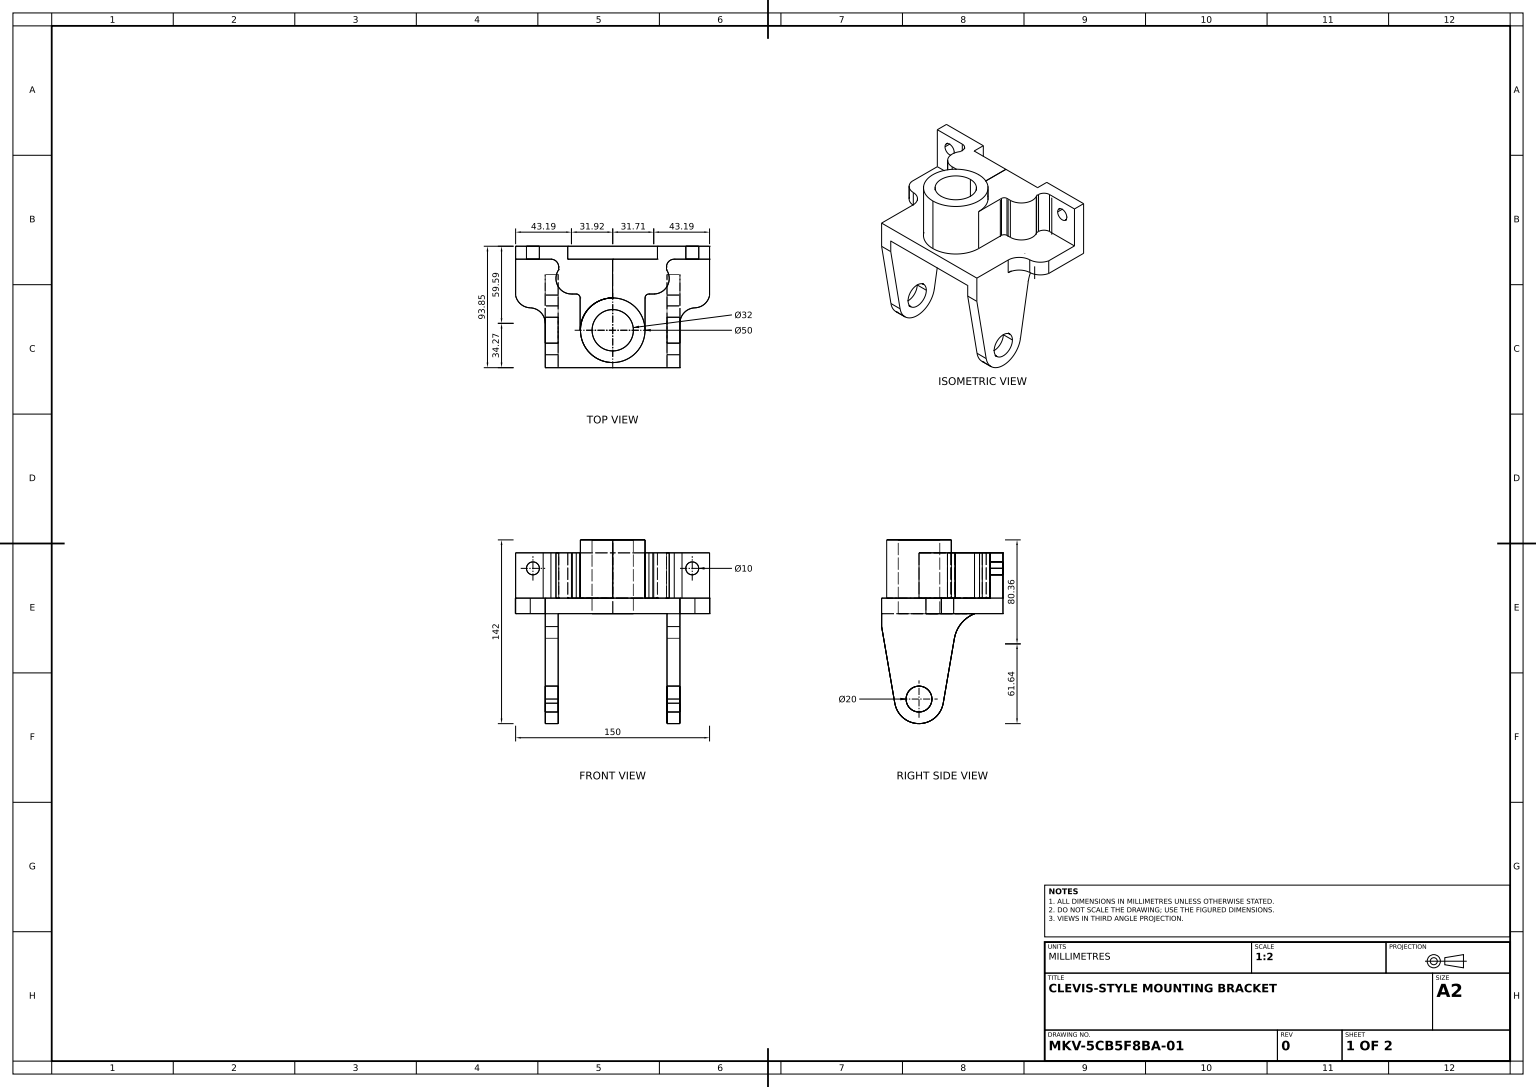
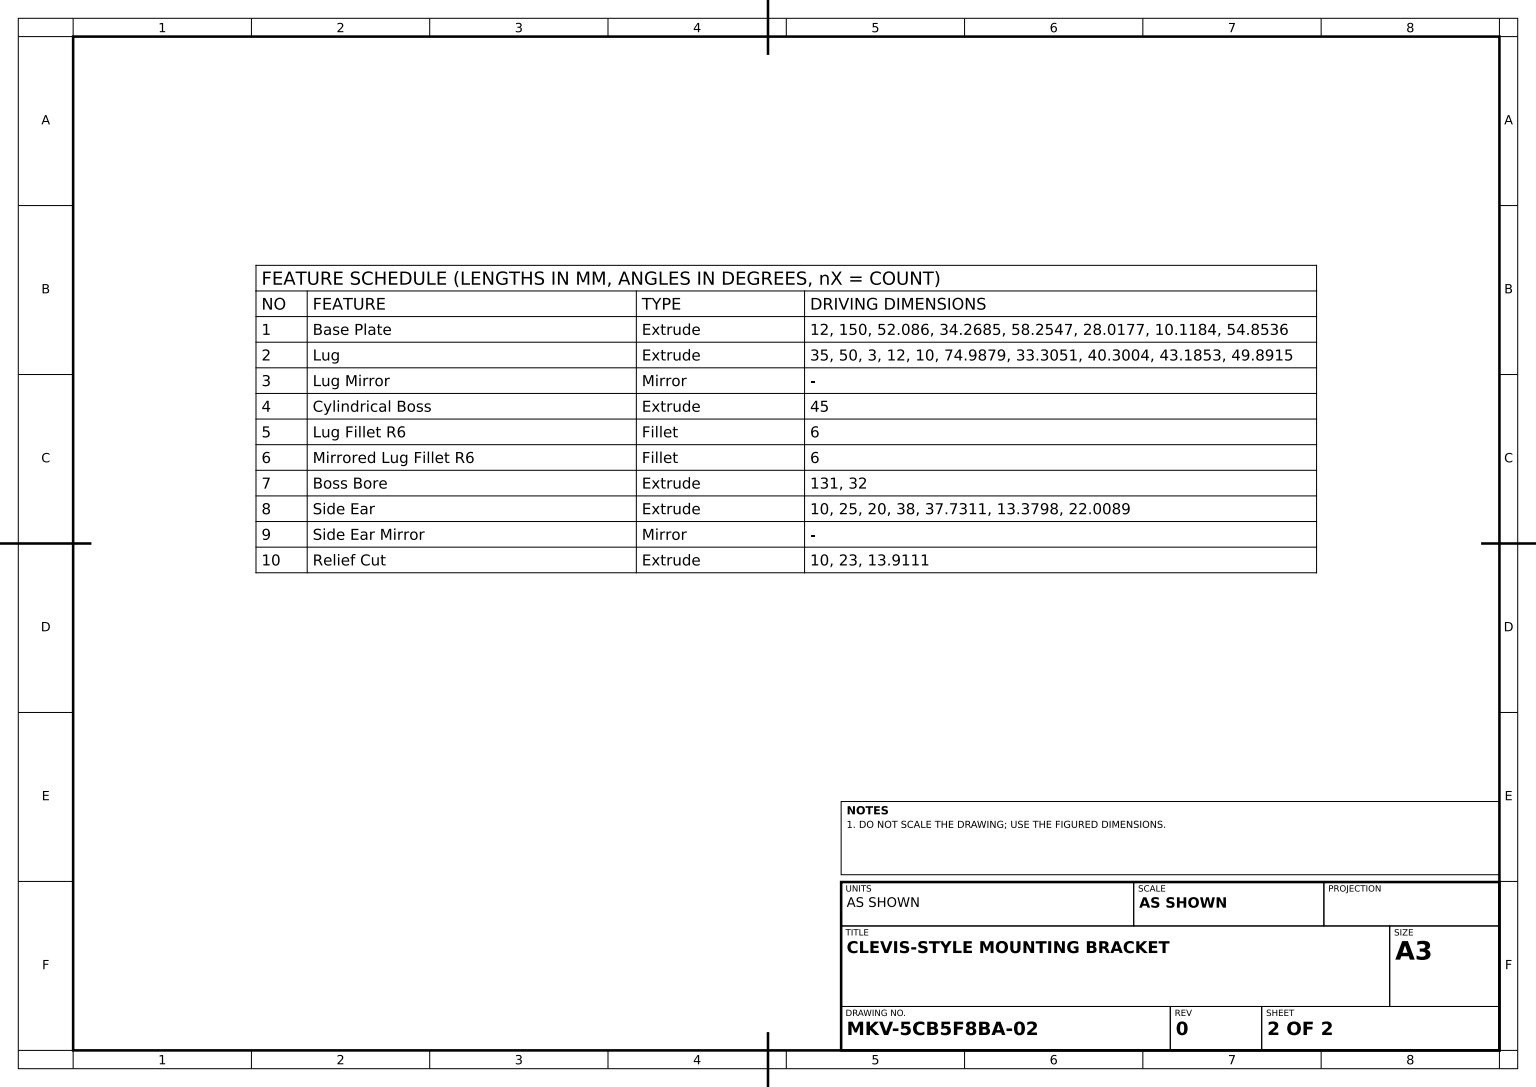
from build123d import *

# Parameters (mm, degrees)
BASE_PLATE_DEPTH         = 12
LUG_DEPTH                = 35
BOSS_SKETCH_R            = 25
CYLINDRICAL_BOSS_DEPTH   = 45
LUG_FILLET_R6_R          = 6
MIRRORED_LUG_FILLET_R6_R = 6
BOSS_BORE_SKETCH_R       = 16
BOSS_BORE_DEPTH          = 131
SIDE_EAR_SKETCH_R        = 10.000000003
SIDE_EAR_DEPTH           = 10
RELIEF_CUT_SKETCH_R      = 5
RELIEF_CUT_DEPTH         = 10


with BuildPart() as part:
    # Base Plate Sketch → Base Plate (new body)
    with BuildSketch(Plane(origin=(0, 0, 0), x_dir=(1, 0, 0), z_dir=(0, 1, 0))):
        with BuildLine():
            Line((0, 0), (52.086042587, 0))
            Line((52.086042587, 0), (52.086042587, 34.268491931))
            ThreePointArc((52.086042587, 34.268491931), (55.457925039, 42.608491187), (63.678640518, 46.261574252))
            ThreePointArc((63.678640518, 46.261574252), (70.963844757, 49.044672415), (75, 55.717699243))
            Line((75, 55.717699243), (75, 83.735383518))
            Line((75, 83.735383518), (75, 93.85377774))
            Line((75, 93.85377774), (20.146433568, 93.85377774))
            Line((20.146433568, 93.85377774), (-75, 93.85377774))
            Line((-75, 93.85377774), (-75, 83.735383518))
            Line((-75, 83.735383518), (-75, 55.717699243))
            ThreePointArc((-75, 55.717699243), (-70.963844757, 49.044672415), (-63.678640518, 46.261574252))
            ThreePointArc((-63.678640518, 46.261574252), (-55.457925039, 42.608491187), (-52.086042587, 34.268491931))
            Line((-52.086042587, 34.268491931), (-52.086042587, 0))
            Line((-52.086042587, 0), (0, 0))
        make_face()
    extrude(amount=BASE_PLATE_DEPTH)

    # Lug Sketch → Lug (add)
    with BuildSketch(Plane(origin=(0, 12, 0), x_dir=(1, 0, 0), z_dir=(0, 1, 0))):
        with BuildLine():
            ThreePointArc((0.048175719, 53.923822509), (17.764829386, 46.622880149), (25.108500916, 28.923895292))
            Line((25.108500916, 28.923895292), (25.108500916, 53.923895292))
            ThreePointArc((25.108500916, 53.923895292), (25.987180573, 56.045215635), (28.108500916, 56.923895292))
            Line((28.108500916, 56.923895292), (31.814716412, 56.923895292))
            ThreePointArc((31.814716412, 56.923895292), (42.43838692, 63.34378553), (41.694924329, 75.734291134))
            Line((41.694924329, 75.734291134), (41.694924329, 83.85377774))
            Line((41.694924329, 83.85377774), (75, 83.85377774))
            Line((75, 83.85377774), (75, 93.85377774))
            Line((75, 93.85377774), (41.694924329, 93.85377774))
            Line((41.694924329, 93.85377774), (34.699589824, 93.85377774))
            Line((34.699589824, 93.85377774), (34.699589824, 83.85377774))
            Line((34.699589824, 83.85377774), (0.012065057, 83.85377774))
            Line((0.012065057, 83.85377774), (0.048175719, 53.923822509))
        make_face()
    lug = extrude(amount=LUG_DEPTH)

    # Lug Mirror: Lug across plane
    add(lug.mirror(Plane(origin=(0, 0, 0), x_dir=(0, 0, 1), z_dir=(1, 0, 0))))

    # Boss Sketch → Cylindrical Boss (add)
    with BuildSketch(Plane(origin=(0, 12, 0), x_dir=(1, 0, 0), z_dir=(0, 1, 0))):
        with Locations(Location((0.108500916, 28.923895292, 0), (0, 0, 90.138255303))):
            Circle(BOSS_SKETCH_R)
    extrude(amount=CYLINDRICAL_BOSS_DEPTH)

    # Lug Fillet R6
    lug_fillet_r6_edges = [part.edges().sort_by_distance(p)[0] for p in [
        (41.694924329, 29.5, -83.85377774),
    ]]
    fillet(lug_fillet_r6_edges, radius=LUG_FILLET_R6_R)

    # Mirrored Lug Fillet R6
    mirrored_lug_fillet_r6_edges = [part.edges().sort_by_distance(p)[0] for p in [
        (-41.694924329, 29.5, -83.85377774),
    ]]
    fillet(mirrored_lug_fillet_r6_edges, radius=MIRRORED_LUG_FILLET_R6_R)

    # Boss Bore Sketch → Boss Bore (cut)
    with BuildSketch(Plane(origin=(0, 57, 0), x_dir=(1, 0, 0), z_dir=(0, 1, 0))):
        with Locations(Location((0.108500916, 28.923895292, 0), (0, 0, 270))):
            Circle(BOSS_BORE_SKETCH_R)
    extrude(amount=-BOSS_BORE_DEPTH, mode=Mode.SUBTRACT)

    # Side Ear Sketch → Side Ear (add)
    with BuildSketch(Plane(origin=(52.086042587, 0, 0), x_dir=(0, 0, -1), z_dir=(1, 0, 0))):
        with BuildLine():
            Line((0, 0), (0, -9.993926671))
            Line((0, -9.993926671), (10.199483508, -69.224345425))
            ThreePointArc((10.199483505, -69.224345426), (28.923895292, -85.000000013), (47.648307078, -69.224345426))
            Line((47.648307075, -69.224345425), (56.277342763, -19.113827886))
            ThreePointArc((56.277342763, -19.113827886), (61.607291904, -7.474858686), (71.999618374, 0))
            Line((71.999618374, 0), (0, 0))
        make_face()
        with Locations((28.923895292, -66.00000001)):
            Circle(SIDE_EAR_SKETCH_R, mode=Mode.SUBTRACT)
    side_ear = extrude(amount=-SIDE_EAR_DEPTH)

    # Side Ear Mirror: Side Ear across plane
    add(side_ear.mirror(Plane(origin=(0, 0, 0), x_dir=(0, 0, 1), z_dir=(1, 0, 0))))

    # Relief Cut Sketch → Relief Cut (cut)
    with BuildSketch(Plane.XY.offset(-83.85377774)):
        with Locations((61.606022049, 35)):
            Circle(RELIEF_CUT_SKETCH_R)
        with Locations(Location((-61.606022049, 35, 0), (0, 0, 180))):
            Circle(RELIEF_CUT_SKETCH_R)
    extrude(amount=-RELIEF_CUT_DEPTH, mode=Mode.SUBTRACT)


solid = part.part
